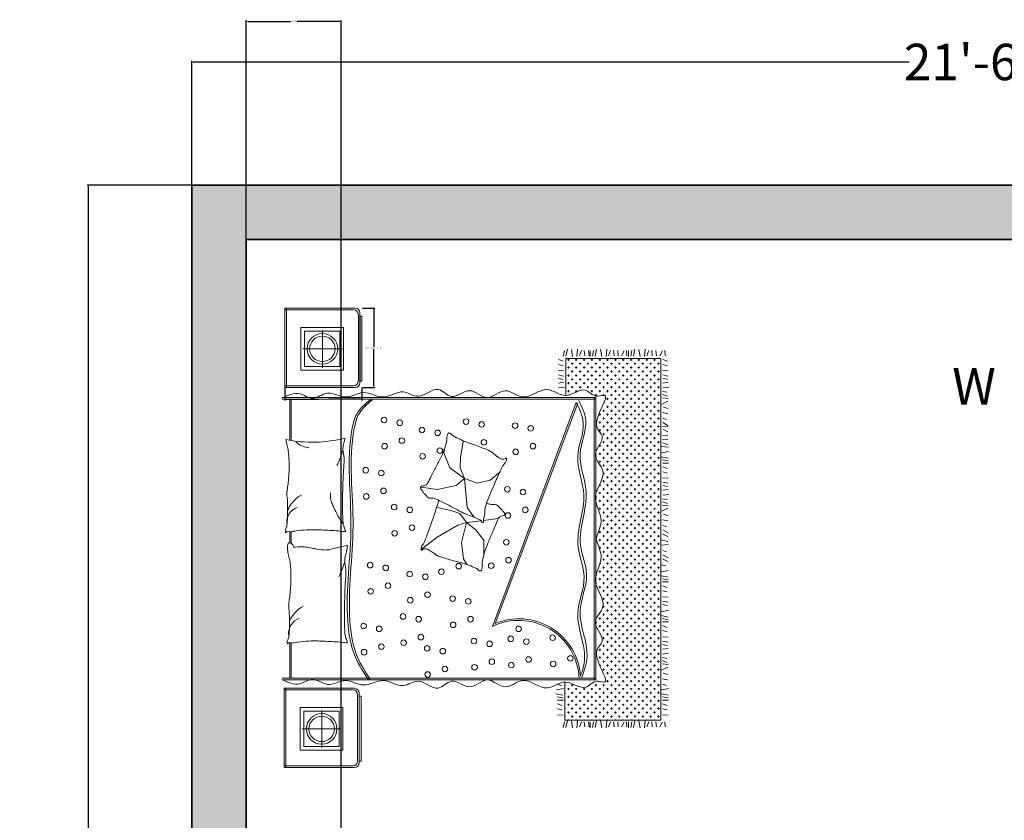
# Model space of a CAD drawing. Units: inches. Extents: x -5 to 330, y -522 to 40.
# Tile 21 of 23: x -5 to 158, y -92 to 40. Entities that reach past the tile are written whole.
import ezdxf

# ---------------------------------------------------------------- set-up
doc = ezdxf.new("R2010")
doc.units = ezdxf.units.IN
doc.header["$MEASUREMENT"] = 0
for name, color, linetype, lineweight in [('A-ANNO-DIMS', 2, 'Continuous', 18), ('A-ANNO-TEXT', 7, 'Continuous', 18), ('A-FURN', 8, 'Continuous', 18), ('A-FURN-PATT', 9, 'Continuous', 13), ('A-WALL', 7, 'Continuous', 35)]:
    doc.layers.add(name, color=color, linetype=linetype, lineweight=lineweight)
doc.layers.add('A-WALL-PATT', color=18, linetype='Continuous', lineweight=13, true_color=0x000000)
doc.styles.get("Standard").update_dxf_attribs({"font": 'arial.ttf'})
doc.dimstyles.get("Standard").update_dxf_attribs({"dimtxt": 0.18, "dimasz": 0.18, "dimexe": 0.18, "dimexo": 0.0625, "dimgap": 0.09, "dimtad": 0, "dimtih": 1, "dimtoh": 1, "dimdec": 0, "dimzin": 0, "dimdsep": 46, "dimlunit": 3, "dimtxsty": 'Standard', "dimcen": 0.09, "dimadec": 0, "dimazin": 0, "dimtfac": 1, "dimtdec": 0, "dimtofl": 0, "dimtmove": 0, "dimatfit": 3, "dimfxl": 1, "dimtolj": 1, "dimtzin": 0, "dimarcsym": 0})

# ---------------------------------------------------------------- blocks, each defined once
blk = doc.blocks.new('*D1')
at = {"layer": 'A-ANNO-DIMS', "color": 0, "lineweight": -2, "transparency": 16777216}
for p, q in [((23.51, 12.42), (23.51, 32.82)), ((23.69, 32.64), (141.81, 32.64)), ((280.83, 32.64), (162.71, 32.64)), ((281.01, 12.42), (281.01, 32.82))]:
    blk.add_line(p, q, dxfattribs=at)
at = {"layer": 'A-ANNO-DIMS', "color": 0, "transparency": 16777216}
for points in [[(23.69, 32.67), (23.69, 32.61), (23.51, 32.64)], [(280.83, 32.67), (280.83, 32.61), (281.01, 32.64)]]:
    blk.add_solid(points, dxfattribs=at)
at = {"layer": 'Defpoints', "color": 0, "transparency": 16777216}
for p in [(281.01, 32.64), (23.51, 12.36), (281.01, 12.36)]:
    blk.add_point(p, dxfattribs=at)
at = {"layer": 'A-ANNO-DIMS', "color": 0, "transparency": 16777216, "insert": (152.26, 32.64), "char_height": 6, "attachment_point": 5}
blk.add_mtext('\\A1;21\'-6"', dxfattribs=at)
blk = doc.blocks.new('*D2')
at = {"layer": 'A-ANNO-DIMS', "color": 0, "lineweight": -2, "transparency": 16777216}
for p, q in [((23.45, 12.36), (6.27, 12.36)), ((6.45, 12.18), (6.45, -203.74)), ((6.45, -425.96), (6.45, -210.05)), ((23.45, -426.14), (6.27, -426.14))]:
    blk.add_line(p, q, dxfattribs=at)
at = {"layer": 'A-ANNO-DIMS', "color": 0, "transparency": 16777216}
for points in [[(6.42, 12.18), (6.48, 12.18), (6.45, 12.36)], [(6.42, -425.96), (6.48, -425.96), (6.45, -426.14)]]:
    blk.add_solid(points, dxfattribs=at)
at = {"layer": 'Defpoints', "color": 0, "transparency": 16777216}
for p in [(23.51, 12.36), (6.45, -426.14), (23.51, -426.14)]:
    blk.add_point(p, dxfattribs=at)
at = {"layer": 'A-ANNO-DIMS', "color": 0, "transparency": 16777216, "insert": (6.45, -206.89), "char_height": 6, "attachment_point": 5}
blk.add_mtext('\\A1;36\'-7"', dxfattribs=at)
blk = doc.blocks.new('NIGHTSTAND-13IN')
for p, q in [((0, 0), (0, 13.05)), ((0, 13.05), (11.58, 13.05)), ((0.26, 0), (0.26, 13.05)), ((0, 12.79), (11.32, 12.79)), ((12.1, 12.01), (12.1, 1.03)), ((12.36, 12.27), (12.36, 0.77)), ((9.67, 9.89), (2.61, 9.89)), ((2.61, 2.83), (2.61, 9.89)), ((9.67, 2.83), (9.67, 9.89)), ((9.04, 9.26), (3.24, 9.26)), ((3.24, 3.46), (3.24, 9.26)), ((6.17, 3.23), (6.17, 9.39)), ((9.04, 3.46), (9.04, 9.26)), ((2.96, 6.35), (9.46, 6.35)), ((9.04, 3.46), (3.24, 3.46)), ((9.67, 2.83), (2.61, 2.83)), ((11.32, 0.26), (0, 0.26)), ((11.58, 0), (0, 0))]:
    blk.add_line(p, q)
blk.add_lwpolyline([(12.38, 11.76), (12.38, 1.04), (12.69, 1.04), (12.69, 11.76)], close=True)
for radius in [2.52, 2.1]:
    blk.add_circle((6.17, 6.35), radius)
for centre, start, end in [((11.58, 12.27), 0, 90), ((11.32, 12.01), 0, 90), ((11.32, 1.03), 270, 0), ((11.58, 0.77), 270, 0)]:
    blk.add_arc(centre, 0.775, start, end)
blk = doc.blocks.new('*D25')
at = {"layer": 'A-ANNO-DIMS', "color": 0, "lineweight": -2, "transparency": 16777216}
for p, q in [((51.65, -7.95), (53.72, -7.95)), ((53.54, -8.13), (53.54, -14.29)), ((53.54, -20.81), (53.54, -14.65)), ((51.65, -20.99), (53.72, -20.99))]:
    blk.add_line(p, q, dxfattribs=at)
at = {"layer": 'A-ANNO-DIMS', "color": 0, "transparency": 16777216}
for points in [[(53.51, -8.13), (53.57, -8.13), (53.54, -7.95)], [(53.51, -20.81), (53.57, -20.81), (53.54, -20.99)]]:
    blk.add_solid(points, dxfattribs=at)
at = {"layer": 'Defpoints', "color": 0, "transparency": 16777216}
for p in [(51.58, -7.95), (53.54, -7.95), (51.58, -20.99)]:
    blk.add_point(p, dxfattribs=at)
at = {"layer": 'A-ANNO-DIMS', "color": 0, "transparency": 16777216, "insert": (53.54, -14.47), "char_height": 0.18, "attachment_point": 5}
blk.add_mtext('\\A1;NIGHTSTAND 1\'-1" TYP.', dxfattribs=at)
blk = doc.blocks.new('*D26')
at = {"layer": 'A-ANNO-DIMS', "color": 0, "lineweight": -2, "transparency": 16777216}
for p, q in [((38.89, -21.05), (38.89, -23.13)), ((51.58, -21.05), (51.58, -23.13)), ((39.07, -22.95), (44.4, -22.95)), ((51.4, -22.95), (46.08, -22.95))]:
    blk.add_line(p, q, dxfattribs=at)
at = {"layer": 'A-ANNO-DIMS', "color": 0, "transparency": 16777216}
for points in [[(39.07, -22.92), (39.07, -22.98), (38.89, -22.95)], [(51.4, -22.92), (51.4, -22.98), (51.58, -22.95)]]:
    blk.add_solid(points, dxfattribs=at)
at = {"layer": 'Defpoints', "color": 0, "transparency": 16777216}
for p in [(38.89, -20.99), (51.58, -20.99), (51.58, -22.95)]:
    blk.add_point(p, dxfattribs=at)
at = {"layer": 'A-ANNO-DIMS', "color": 0, "transparency": 16777216, "insert": (45.24, -22.95), "char_height": 0.18, "attachment_point": 5}
blk.add_mtext('\\A1;1\'-0 1/2" TYP.', dxfattribs=at)
blk = doc.blocks.new('*D43')
at = {"layer": 'A-ANNO-DIMS', "color": 0, "lineweight": -2, "transparency": 16777216}
for p, q in [((32.51, -297.08), (32.51, 39.52)), ((32.69, 39.34), (39.79, 39.34)), ((47.95, 39.34), (40.85, 39.34)), ((48.13, -297.08), (48.13, 39.52))]:
    blk.add_line(p, q, dxfattribs=at)
at = {"layer": 'A-ANNO-DIMS', "color": 0, "transparency": 16777216}
for points in [[(32.69, 39.37), (32.69, 39.31), (32.51, 39.34)], [(47.95, 39.37), (47.95, 39.31), (48.13, 39.34)]]:
    blk.add_solid(points, dxfattribs=at)
at = {"layer": 'Defpoints', "color": 0, "transparency": 16777216}
for p in [(48.13, 39.34), (32.51, -297.14), (48.13, -297.14)]:
    blk.add_point(p, dxfattribs=at)
at = {"layer": 'A-ANNO-DIMS', "color": 0, "transparency": 16777216, "insert": (40.32, 39.34), "char_height": 0.18, "attachment_point": 5}
blk.add_mtext('\\A1;1\'-3 1/2"', dxfattribs=at)

msp = doc.modelspace()

# ---------------------------------------------------------------- hatches: boundary and pattern name
at = {"layer": 'A-FURN-PATT'}
h = msp.add_hatch(dxfattribs=at)
h.set_pattern_fill('CROSS', color=256, scale=2.58433, angle=-90, style=0)
h.set_pattern_definition([(270, (2.9259, -5613.9358), (0.64608249, -0.64608249), [0.32304124, -0.96912373]), (360, (2.7644, -5614.09734), (0.64608249, 0.64608249), [0.32304124, -0.96912373])])
edge = h.paths.add_edge_path()
edge.add_line((100.87, -75.84), (85.03, -75.84))
edge.add_line((85.03, -75.84), (85.03, -69.58))
edge.add_spline(control_points=[(85.03, -69.58), (85.08, -69.58), (86.28, -69.56), (88.27, -71.42), (89.86, -69.09), (93.41, -70.4), (88.82, -65.04), (91.96, -62.62), (90.37, -61.1), (90.13, -60.18)], knot_values=[1896.039366, 1896.039366, 1896.039366, 1896.039366, 1901.133447, 2037.052147, 2110.507177, 2158.377997, 2368.992723, 2430.676444, 2542.061162, 2542.061162, 2542.061162, 2542.061162], degree=3, periodic=0)
edge.add_line((90.13, -60.18), (90.13, -59.44))
edge.add_spline(control_points=[(90.13, -59.44), (90.34, -58.65), (92.37, -56.72), (90.41, -54.57), (90.13, -53.24)], knot_values=[2572.217644, 2572.217644, 2572.217644, 2572.217644, 2670.523569, 2827.764492, 2827.764492, 2827.764492, 2827.764492], degree=3, periodic=0)
edge.add_line((90.13, -53.24), (90.13, -52.16))
edge.add_spline(control_points=[(90.13, -52.16), (90.33, -51.08), (91.68, -49), (90.44, -46.95), (90.18, -45.95)], knot_values=[2870.498313, 2870.498313, 2870.498313, 2870.498313, 2999.108306, 3118.80064, 3118.80064, 3118.80064, 3118.80064], degree=3, periodic=0)
edge.add_spline(control_points=[(90.18, -45.95), (90.44, -44.95), (91.68, -42.9), (90.33, -40.82), (90.13, -39.74)], knot_values=[2870.498313, 2870.498313, 2870.498313, 2870.498313, 2990.190647, 3118.80064, 3118.80064, 3118.80064, 3118.80064], degree=3, periodic=0)
edge.add_line((90.13, -39.74), (90.13, -38.66))
edge.add_spline(control_points=[(90.13, -38.66), (90.41, -37.33), (92.37, -35.17), (90.34, -33.24), (90.13, -32.46)], knot_values=[2572.217644, 2572.217644, 2572.217644, 2572.217644, 2729.458567, 2827.764492, 2827.764492, 2827.764492, 2827.764492], degree=3, periodic=0)
edge.add_line((90.13, -32.46), (90.13, -31.72))
edge.add_spline(control_points=[(90.13, -31.72), (90.37, -30.79), (91.96, -29.28), (88.82, -26.86), (93.41, -21.5), (89.86, -22.8), (88.28, -20.49), (86.36, -22.27), (85.2, -22.32)], knot_values=[1902.697505, 1902.697505, 1902.697505, 1902.697505, 2014.082222, 2075.765943, 2286.38067, 2334.251489, 2407.70652, 2542.061162, 2542.061162, 2542.061162, 2542.061162], degree=3, periodic=0)
edge.add_line((85.2, -22.32), (85.2, -16.25))
edge.add_line((85.2, -16.25), (100.87, -16.25))
edge.add_line((100.87, -16.25), (100.87, -75.84))
at = {"layer": 'A-WALL-PATT'}
h = msp.add_hatch(color=256, dxfattribs=at)
h.dxf.hatch_style = 1
h.paths.add_polyline_path([(164.01, -44.15), (159.51, -44.15), (159.51, -153.14), (164.01, -153.14)], flags=17)
h.paths.add_polyline_path([(224.01, -188.14), (272.01, -188.14), (272.01, -218.14), (260.01, -218.14), (260.01, -222.64), (272.01, -222.64), (272.01, -292.64), (159.01, -292.64), (159.01, -297.14), (272.01, -297.14), (272.01, -417.14), (245.51, -417.14), (245.51, -426.14), (272.01, -426.14), (272.01, -495.14), (281.01, -495.14), (281.01, 12.36), (23.51, 12.36), (23.51, -426.14), (62.92, -426.14), (62.92, -417.14), (32.51, -417.14), (32.51, -297.14), (48.13, -297.14), (48.13, -292.64), (32.51, -292.64), (32.51, -140.64), (133.51, -140.64), (133.51, -131.64), (32.51, -131.64), (32.51, 3.36), (159.51, 3.36), (164.01, 3.36), (220.01, 3.36), (224.51, 3.36), (272.01, 3.36), (272.01, -179.14), (159.51, -179.14), (159.51, -188.14), (219.51, -188.14), (219.51, -266.64), (224.01, -266.64), (224.01, -222.64), (236.01, -222.64), (236.01, -218.14), (224.01, -218.14)])
h.paths.add_polyline_path([(133.01, -292.64), (128.51, -292.64), (128.51, -297.14), (128.51, -417.14), (122.92, -417.14), (122.92, -426.14), (133.01, -426.14)], flags=17)
h.paths.add_polyline_path([(185.51, -417.14), (159.01, -417.14), (159.01, -426.14), (185.51, -426.14)], flags=17)
h.paths.add_polyline_path([(133.51, -140.64), (129.01, -140.64), (129.01, -246.64), (133.51, -246.64)], flags=17)
h.paths.add_polyline_path([(246.01, -48.64), (224.51, -48.64), (224.51, -27.63), (220.01, -27.63), (220.01, -48.64), (198.6, -48.64), (198.6, -53.14), (246.01, -53.14)], flags=17)

# ---------------------------------------------------------------- linework, layer by layer
at = {"layer": 'A-FURN'}
for p, q in [((84.79, -15.84), (84.97, -14.9)), ((85.21, -15.84), (85.46, -14.69)), ((86.31, -15.91), (86.12, -14.76)), ((87.04, -15.91), (87.15, -14.69)), ((87.43, -15.77), (87.77, -14.9)), ((88.33, -15.77), (88.25, -14.9)), ((89.03, -15.77), (88.94, -14.9)), ((89.24, -15.91), (89.24, -14.94)), ((89.61, -15.84), (89.79, -14.9)), ((90.03, -15.84), (90.28, -14.69)), ((91.13, -15.91), (90.94, -14.76)), ((91.85, -15.91), (91.97, -14.69)), ((92.25, -15.77), (92.58, -14.9)), ((93.15, -15.77), (93.07, -14.9)), ((93.84, -15.77), (93.76, -14.9)), ((94.38, -15.77), (94.83, -14.97)), ((95.28, -15.77), (95.2, -14.9)), ((95.55, -15.91), (95.55, -14.94)), ((95.92, -15.84), (96.1, -14.9)), ((96.34, -15.84), (96.59, -14.69)), ((97.44, -15.91), (97.25, -14.76)), ((98.16, -15.91), (98.28, -14.69)), ((98.56, -15.77), (98.89, -14.9)), ((99.46, -15.77), (99.38, -14.9)), ((100.15, -15.77), (100.07, -14.9)), ((100.69, -15.77), (101.14, -14.97)), ((101.59, -15.77), (101.51, -14.9)), ((84.75, -16.7), (83.99, -16.4)), ((84.75, -17.43), (83.99, -17.23)), ((85.2, -16.25), (100.87, -16.25)), ((85.2, -22.32), (85.2, -16.25)), ((100.87, -16.25), (100.87, -75.84)), ((101.96, -16.7), (101.2, -16.4)), ((101.96, -17.43), (101.2, -17.23)), ((84.89, -18.28), (83.99, -18.23)), ((84.82, -19.12), (83.99, -18.95)), ((102.1, -18.28), (101.2, -18.23)), ((102.03, -19.12), (101.2, -18.95)), ((84.75, -19.68), (83.99, -19.5)), ((84.89, -20.16), (83.99, -20.28)), ((84.96, -20.95), (83.99, -21.09)), ((101.96, -19.68), (101.2, -19.5)), ((102.1, -20.16), (101.2, -20.28)), ((102.17, -20.95), (101.2, -21.09)), ((38.44, -22.69), (90.13, -22.69)), ((89.87, -22.69), (89.87, -69.21)), ((90.13, -22.69), (90.13, -69.21)), ((101.89, -21.8), (101.16, -21.67)), ((101.96, -22.46), (101.16, -22.16)), ((102.1, -22.83), (101.16, -22.71)), ((38.44, -22.95), (90.13, -22.95)), ((39.67, -22.95), (39.67, -29.73)), ((39.93, -22.95), (39.93, -29.77)), ((86.93, -23.48), (73.09, -60.41)), ((87.17, -23.57), (73.55, -59.92)), ((102.03, -23.25), (101.02, -23.74)), ((102.1, -24.47), (101.3, -24.23)), ((102.02, -25.33), (101.17, -25.14)), ((102.02, -27.43), (101.16, -27.51)), ((101.83, -26.29), (101.2, -26.08)), ((102.1, -27.31), (101.2, -26.8)), ((102.02, -28.87), (101.16, -28.95)), ((102.02, -28.33), (101.23, -27.88)), ((67.85, -32.49), (68.29, -29.96)), ((68.29, -29.96), (68.46, -29.87)), ((102.16, -30.86), (100.94, -30.74)), ((102.02, -29.56), (101.16, -29.64)), ((102.02, -30.46), (101.16, -30.13)), ((65.09, -31.78), (65.18, -31.16)), ((66.07, -34.23), (65.09, -31.78)), ((102.09, -32.68), (100.94, -32.43)), ((102.16, -31.58), (101.01, -31.77)), ((67.76, -34.27), (67.85, -32.49)), ((102.09, -33.1), (101.16, -32.92)), ((102.16, -33.47), (101.2, -33.47)), ((101.96, -34.38), (101.2, -34.08)), ((68.47, -36.01), (66.07, -34.23)), ((68.47, -36.01), (67.76, -34.27)), ((72.74, -36.27), (74.35, -34.89)), ((101.96, -35.11), (101.2, -34.91)), ((63.98, -37.83), (67.14, -37.16)), ((67.14, -37.16), (68.47, -36.01)), ((68.47, -36.01), (68.96, -40.81)), ((68.47, -36.01), (70.6, -36.81)), ((70.6, -36.81), (72.74, -36.27)), ((102.1, -35.96), (101.2, -35.91)), ((102.03, -36.8), (101.2, -36.63)), ((101.96, -37.36), (101.2, -37.18)), ((61.32, -37.47), (63.98, -37.83)), ((102.1, -37.84), (101.2, -37.96)), ((102.17, -38.63), (101.2, -38.77)), ((101.89, -39.48), (101.16, -39.36)), ((101.96, -40.14), (101.16, -39.84)), ((102.1, -40.51), (101.16, -40.39)), ((66.25, -41.28), (63.96, -40.77)), ((67.74, -41.79), (66.25, -41.28)), ((68.81, -43.27), (67.74, -41.79)), ((68.45, -41.77), (69.91, -42.36)), ((68.96, -40.81), (69.89, -42.1)), ((69.89, -42.1), (70.11, -42.41)), ((102.03, -40.93), (101.02, -41.42)), ((102.1, -42.15), (101.3, -41.91)), ((64.01, -45.67), (67.38, -43.73)), ((67.38, -43.73), (68.81, -43.27)), ((68.81, -43.27), (67.99, -46.59)), ((68.81, -43.27), (71.24, -42.97)), ((68.81, -43.27), (70.44, -44.55)), ((69.91, -42.36), (71.03, -42.82)), ((71.62, -42.92), (74.06, -42.62)), ((102.02, -43.01), (101.17, -42.82)), ((101.83, -43.97), (101.2, -43.76)), ((39.67, -44.8), (39.67, -46.6)), ((39.93, -44.8), (39.93, -46.7)), ((70.44, -44.55), (71.67, -46.24)), ((102.02, -45.58), (101.16, -45.18)), ((102.1, -44.99), (101.2, -44.48)), ((49.14, -47.02), (48.36, -47.21)), ((61.32, -47.72), (64.01, -45.67)), ((67.99, -46.59), (68.35, -49.25)), ((71.67, -46.24), (71.67, -48.64)), ((102.03, -46.39), (100.95, -46.14)), ((102.1, -46.87), (101.02, -46.99)), ((48.36, -47.21), (46.23, -47.74)), ((101.83, -48.08), (101.2, -47.86)), ((102.1, -49.09), (101.2, -48.59)), ((68.35, -49.25), (68.87, -50.18)), ((101.68, -50.41), (100.95, -50.25)), ((102.02, -49.69), (101.16, -49.28)), ((102.13, -51.19), (100.98, -51.38)), ((102.06, -52.28), (100.91, -52.04)), ((102.06, -52.7), (101.12, -52.53)), ((102.13, -53.07), (101.16, -53.07)), ((101.93, -53.99), (101.16, -53.68)), ((101.93, -54.71), (101.16, -54.51)), ((102.07, -55.56), (101.16, -55.51)), ((102, -56.41), (101.16, -56.24)), ((101.93, -56.96), (101.16, -56.78)), ((102.13, -57.77), (100.98, -57.96)), ((102.06, -58.86), (100.91, -58.62)), ((102.06, -59.29), (101.12, -59.11)), ((102.13, -59.65), (101.16, -59.65)), ((101.93, -60.57), (101.16, -60.27)), ((101.93, -61.3), (101.16, -61.09)), ((39.67, -63.05), (39.67, -68.95)), ((39.93, -63.12), (39.93, -68.95)), ((102.07, -62.14), (101.16, -62.1)), ((102, -62.99), (101.16, -62.82)), ((101.93, -63.54), (101.16, -63.37)), ((102.07, -64.02), (101.16, -64.15)), ((102.14, -64.81), (101.16, -64.95)), ((101.86, -65.67), (101.12, -65.54)), ((101.93, -66.33), (101.12, -66.02)), ((102, -67.12), (100.99, -67.61)), ((102.07, -66.69), (101.12, -66.57)), ((102.07, -68.34), (101.27, -68.09)), ((38.44, -68.95), (90.13, -68.95)), ((38.44, -69.21), (90.13, -69.21)), ((85.03, -75.84), (85.03, -69.58)), ((101.99, -69.2), (101.13, -69.01)), ((84.8, -70.65), (83.65, -70.83)), ((84.47, -70.16), (83.84, -69.94)), ((102.13, -70.65), (100.98, -70.83)), ((101.79, -70.16), (101.16, -69.94)), ((84.73, -71.74), (83.58, -71.49)), ((84.73, -72.16), (83.8, -71.99)), ((84.8, -72.53), (83.84, -72.53)), ((102.06, -71.74), (100.91, -71.49)), ((102.06, -72.16), (101.12, -71.99)), ((102.13, -72.53), (101.16, -72.53)), ((84.61, -73.44), (83.84, -73.14)), ((84.61, -74.17), (83.84, -73.97)), ((101.93, -73.44), (101.16, -73.14)), ((101.93, -74.17), (101.16, -73.97)), ((84.74, -75.02), (83.84, -74.97)), ((84.79, -77.03), (84.97, -76.1)), ((100.87, -75.84), (85.03, -75.84)), ((85.21, -77.03), (85.46, -75.88)), ((86.31, -77.1), (86.12, -75.95)), ((87.04, -77.1), (87.15, -75.88)), ((87.43, -76.96), (87.77, -76.1)), ((88.33, -76.96), (88.25, -76.1)), ((89.03, -76.96), (88.94, -76.1)), ((89.24, -77.1), (89.24, -76.14)), ((89.61, -77.03), (89.79, -76.1)), ((90.03, -77.03), (90.28, -75.88)), ((91.13, -77.1), (90.94, -75.95)), ((91.85, -77.1), (91.97, -75.88)), ((92.25, -76.96), (92.58, -76.1)), ((93.15, -76.96), (93.07, -76.1)), ((93.84, -76.96), (93.76, -76.1)), ((94.38, -76.96), (94.83, -76.17)), ((95.28, -76.96), (95.2, -76.1)), ((95.55, -77.1), (95.55, -76.14)), ((95.92, -77.03), (96.1, -76.1)), ((96.34, -77.03), (96.59, -75.88)), ((97.44, -77.1), (97.25, -75.95)), ((98.16, -77.1), (98.28, -75.88)), ((98.56, -76.96), (98.89, -76.1)), ((99.46, -76.96), (99.38, -76.1)), ((100.15, -76.96), (100.07, -76.1)), ((100.69, -76.96), (101.14, -76.17)), ((102.07, -75.02), (101.16, -74.97)), ((101.59, -76.96), (101.51, -76.1))]:
    msp.add_line(p, q, dxfattribs=at)
for centre in [(55.23, -26.37), (57.81, -26.83), (61.48, -28.02), (68.75, -26.64), (71.32, -27.1), (76.84, -27.29), (79.41, -27.75), (64.06, -28.48), (55.32, -30.69), (58.17, -29.77), (71.69, -30.05), (79.78, -30.69), (61.58, -32.35), (64.43, -31.43), (76.93, -31.61), (52.2, -34.65), (54.77, -35.11), (75.57, -37.79), (52.29, -38.97), (55.14, -38.05), (78.14, -38.25), (56.89, -40.72), (59.46, -41.18), (75.66, -42.11), (78.51, -41.19), (59.83, -44.12), (56.98, -45.04), (75.39, -46.53), (52.93, -50.29), (55.51, -50.75), (67.53, -50.46), (72.9, -50.39), (75.75, -49.47), (59.46, -51.76), (62.04, -52.22), (64.68, -51.38), (55.88, -53.69), (53.03, -54.61), (62.4, -55.16), (59.55, -56.08), (66.54, -55.81), (69.11, -56.27), (58.36, -58.75), (51.85, -60.33), (60.93, -59.21), (66.63, -60.13), (69.48, -59.21), (54.43, -60.79), (61.3, -62.16), (77.41, -60.79), (54.79, -63.73), (58.45, -63.08), (70.05, -62.81), (72.63, -63.27), (76.12, -62.44), (78.7, -62.9), (83.02, -62.26), (51.94, -64.65), (62.33, -64.01), (64.91, -64.47), (73, -66.21), (76.21, -66.77), (79.06, -65.85), (83.11, -66.58), (85.96, -65.66), (62.42, -68.33), (65.27, -67.41), (70.15, -67.13)]:
    msp.add_circle(centre, 0.46, dxfattribs=at)
for centre, radius, start, end in [((67.14, -29.31), 1.55, 166.9598, 183.3881), ((66.91, -29.26), 1.32, 148.3083, 166.9598), ((65.92, -28.65), 0.15, 90.9614, 148.3083), ((65.92, -28.93), 0.433, 40.5086, 90.9614), ((67.74, -27.38), 1.95, 220.5086, 243.6668), ((97.39, 32.52), 68.79, 243.6668, 244.8268), ((43.36, -7.71), 22.32, 258.8097, 284.0422), ((46.82, -28.45), 7.88, 188.4372, 195.744), ((33.22, -32.29), 6.26, 7.5469, 15.744), ((43.22, -27.37), 3.62, 224.9024, 264.3689), ((52.21, -31.16), 3.77, 173.5659, 191.5586), ((51.54, -31.09), 3.09, 162.6136, 173.5659), ((42.92, -28.39), 5.94, 342.6136, 350.5159), ((54.71, -27.42), 11.11, 339.2514, 347.3748), ((63.97, -29.5), 1.63, 347.3748, 3.3881), ((70.1, -25.53), 4.65, 244.8268, 249.2919), ((73.44, -16.69), 14.1, 249.2919, 251.7631), ((55.7, -70.53), 42.59, 70.3416, 71.7631), ((52.62, -79.17), 51.76, 67.7645, 70.3416), ((21.93, -33.78), 17.64, 0, 7.5469), ((30.21, -25.72), 19.09, 334.6889, 342.8018), ((42.69, -33.11), 5.95, 357.2509, 11.5586), ((50.03, -25.65), 16.12, 332.5079, 339.2514), ((70.28, -35.95), 5.08, 59.5306, 67.7645), ((71.8, -33.38), 2.09, 45.9036, 59.5306), ((76.74, -28.28), 5.01, 225.9036, 234.6985), ((79.1, -24.94), 9.1, 234.6985, 238.7862), ((12.47, -33.78), 27.11, 353.9133, 0), ((12.37, -31.65), 36.3, 355.3824, 357.2509), ((203.32, -107.58), 157.69, 152.1518, 152.5001), ((-69.51, 36.56), 150.88, 332.1518, 332.5079), ((94.03, -43.87), 21.63, 152.8972, 155.4754), ((74.92, -31.85), 1.02, 238.7862, 251.0332), ((74.71, -32.44), 0.395, 251.0332, 268.3327), ((74.76, -30.84), 1.99, 268.3327, 276.0115), ((76.6, -34.94), 2.05, 137.0187, 152.8972), ((74.93, -32.46), 0.366, 276.0115, 319.0249), ((73.96, -32.49), 1.55, 317.0187, 335.2589), ((75.33, -32.81), 0.163, 72.3233, 139.0249), ((75.34, -32.76), 0.115, 359.5525, 72.3233), ((74.55, -32.76), 0.911, 335.2589, 359.5525), ((135.29, -39.63), 86.89, 177.3904, 179.0296), ((79.89, -37.11), 31.44, 175.3824, 177.3904), ((-8.68, -0.04), 80.04, 332.7098, 333.5853), ((109.67, -58.83), 52.11, 152.5001, 153.5853), ((194.13, -89.53), 131.65, 155.4754, 156.5205), ((25.82, -35.21), 13.68, 349.8101, 353.9133), ((61.55, -37.57), 0.329, 86.7545, 218.8136), ((61.63, -36.32), 0.927, 266.7545, 332.7098), ((147.92, -69.46), 81.28, 156.5205, 158.9957), ((43.16, -38.33), 3.94, 169.8101, 177.4614), ((46.7, -38.48), 7.49, 177.4614, 184.8018), ((43.62, -43.54), 5.17, 113.0028, 118.3168), ((53.42, -38.83), 7.03, 176.4448, 184.0828), ((196.17, -40.66), 147.79, 179.0296, 180.2865), ((62.7, -36.65), 1.8, 218.8136, 224.1274), ((60.57, -38.72), 1.17, 37.5287, 44.1274), ((53.66, -44.03), 9.89, 36.2163, 37.5287), ((75.4, -28.1), 17.07, 216.2163, 217.2151), ((66.29, -35.02), 5.62, 217.2151, 223.5224), ((63.66, -37.52), 2, 223.5224, 234.1064), ((16.76, -41), 22.57, 0.5757, 4.8018), ((41.36, -41.57), 1.98, 141.6114, 152.7604), ((47.74, -46.62), 10.12, 136.1885, 141.6114), ((44.64, -43.64), 5.82, 129.0349, 136.1885), ((41.77, -40.11), 1.27, 118.3168, 129.0349), ((47.9, -39.22), 1.5, 184.0828, 200.6743), ((58.75, -35.13), 13.09, 200.6743, 204.3265), ((80.55, -25.28), 37.01, 204.3265, 206.4985), ((62.83, -38.67), 0.584, 234.1064, 278.0492), ((63.08, -40.42), 1.18, 67.5838, 98.0492), ((-13.74, -16.68), 81.28, 340.9164, 343.3915), ((53.62, -63.34), 25.98, 64.9471, 67.5838), ((61.26, -39.05), 3.01, 343.3915, 349.2634), ((46.16, -79.29), 43.59, 62.9116, 64.9471), ((47.6, -76.5), 40.45, 60.064, 62.9116), ((74.86, -41.41), 3.01, 158.9957, 171.8784), ((80.75, -15.56), 25.98, 250.6552, 251.9797), ((73.08, -39.14), 1.18, 251.9797, 282.4451), ((73.46, -40.87), 0.584, 58.5023, 102.4451), ((72.72, -42.08), 2, 47.9183, 58.5023), ((41.73, -43.2), 2.56, 108.4397, 184.2159), ((0.71, -41.16), 38.62, 358.0921, 0.5757), ((44.98, -43.43), 6.05, 152.7604, 159.1397), ((54.65, -38.19), 8.08, 206.4985, 212.135), ((78.47, -41.25), 30.08, 180.2865, 183.574), ((70.55, -36.64), 5.54, 240.064, 247.7645), ((67.26, -41.13), 4.64, 345.1193, 352.3216), ((70.03, -41.51), 1.84, 352.3216, 4.5118), ((73.57, -41.23), 1.71, 171.8784, 184.5118), ((74.84, -43.12), 0.927, 91.1504, 157.1056), ((70.29, -44.77), 5.62, 41.611, 47.9183), ((61.74, -52.37), 17.07, 40.6122, 41.611), ((82.2, -34.82), 9.89, 220.6122, 221.9246), ((74.82, -41.86), 0.329, 271.1504, 43.2095), ((75.71, -40.65), 1.17, 221.9246, 228.5233), ((73.75, -42.87), 1.8, 43.2095, 48.5233), ((37.84, -43.56), 1.39, 329.3487, 354.7408), ((18.1, -41.74), 21.21, 354.7408, 358.0921), ((63.76, -32.47), 18.83, 212.135, 215.8263), ((52.21, -42.89), 3.77, 183.574, 192.869), ((49.68, -43.47), 1.17, 192.869, 207.2841), ((-61.35, -0.21), 131.65, 339.8713, 340.9164), ((70.8, -43.37), 0.596, 17.1867, 67.7645), ((71.49, -43.16), 0.121, 197.1867, 340.6201), ((71.38, -43.12), 0.238, 340.6201, 4.2593), ((72.49, -43.04), 0.878, 172.0178, 184.2593), ((76.62, -43.62), 5.05, 165.1193, 172.0178), ((147.73, -73.9), 80.04, 157.1056, 157.9812), ((39.68, -44.65), 0.746, 149.3487, 184.3025), ((39.58, -44.65), 0.649, 184.3025, 201.7883), ((39.06, -44.86), 0.0884, 201.7883, 250.436), ((39.05, -44.89), 0.0599, 250.436, 11.8931), ((39.22, -44.85), 0.111, 111.9904, 191.8931), ((39.33, -45.12), 0.403, 68.579, 111.9904), ((39.78, -43.96), 0.847, 248.579, 278.1335), ((39, -38.51), 6.36, 278.1335, 282.1095), ((41.41, -49.73), 5.13, 97.6809, 102.1095), ((43.88, -68.04), 23.6, 93.3687, 97.6809), ((43.53, -61.99), 17.54, 88.3669, 93.3687), ((43.02, -79.73), 35.28, 86.945, 88.3669), ((26.12, -396.38), 352.39, 86.4951, 86.945), ((47.16, -52.94), 8.3, 80.0016, 86.4951), ((48.68, -44.27), 0.5, 260.0016, 286.6978), ((46.87, -44.92), 1.98, 16.2212, 27.2841), ((46.61, -44.99), 2.26, 7.1204, 16.2212), ((48.82, -44.72), 0.0341, 286.6978, 7.1204), ((-71.9, 17.08), 157.69, 336.5477, 336.896), ((25.22, -24.35), 52.11, 336.896, 337.9812), ((41.63, -47.33), 2.34, 168.7276, 180), ((39.67, -46.94), 0.339, 63.4195, 168.7276), ((39.43, -47.42), 0.883, 4.4002, 63.4195), ((42.19, -46.54), 7, 350.5159, 355.9171), ((49.14, -47.04), 0.0237, 355.9171, 104.0449), ((62.83, -47.88), 1.55, 141.4146, 159.6548), ((60.02, -45.64), 2.05, 321.4146, 337.2931), ((41.95, -38.08), 21.63, 337.2931, 339.8713), ((87.22, -52.86), 16.12, 156.9038, 163.6473), ((211.18, -105.73), 150.88, 156.5477, 156.9038), ((43.46, -47.33), 4.16, 180, 188.4372), ((47.13, -46.78), 7.88, 188.4372, 195.744), ((41.68, -59.99), 12.71, 90, 96.2324), ((41.68, -52.55), 5.27, 80.3156, 90), ((38.73, -69.82), 22.79, 77.8016, 80.3156), ((45.28, -39.53), 8.2, 257.8016, 261.9949), ((46.51, -30.79), 17.03, 261.9949, 267.3351), ((45.8, -46.05), 1.75, 267.3351, 284.0452), ((51.85, -49.42), 3.09, 162.6136, 173.5659), ((43.23, -46.72), 5.94, 342.6136, 350.5159), ((61.45, -47.67), 0.163, 183.9524, 323.4208), ((62.23, -47.66), 0.911, 159.6548, 183.9484), ((61.87, -47.98), 0.366, 100.4074, 143.4208), ((62.17, -49.58), 1.99, 92.7286, 100.4074), ((62.09, -47.99), 0.395, 75.4291, 92.7286), ((61.93, -48.59), 1.02, 63.1821, 75.4291), ((58.29, -55.8), 9.1, 59.0944, 63.1821), ((60.39, -52.29), 5.01, 50.2995, 59.0944), ((64.93, -46.83), 2.09, 230.2995, 243.9265), ((66.24, -44.15), 5.08, 243.9265, 252.1604), ((82.42, -51.46), 11.11, 163.6473, 171.7707), ((33.52, -50.62), 6.26, 7.5469, 15.744), ((22.24, -52.11), 17.64, 0, 7.5469), ((30.52, -44.05), 19.09, 334.6889, 342.8018), ((52.52, -49.49), 3.77, 173.5659, 191.5586), ((43, -51.44), 5.95, 357.2509, 11.5586), ((80.54, 0.3), 51.76, 252.1604, 254.7375), ((78.13, -8.55), 42.59, 254.7375, 256.159), ((64.56, -63.59), 14.1, 73.6878, 76.159), ((67.22, -54.52), 4.65, 69.2227, 73.6878), ((44.46, -114.5), 68.79, 68.0627, 69.2227), ((73.03, -50.1), 1.63, 171.7707, 187.784), ((69.88, -50.53), 1.55, 351.3557, 7.784), ((12.68, -49.98), 36.3, 355.3824, 357.2509), ((69.43, -52.5), 1.95, 44.9045, 68.0627), ((71.12, -50.82), 0.433, 224.9045, 275.3572), ((71.15, -51.1), 0.15, 275.3572, 332.7041), ((70.11, -50.56), 1.32, 332.7041, 351.3557), ((12.77, -52.11), 27.11, 353.9133, 0), ((80.2, -55.44), 31.44, 175.3824, 177.3904), ((26.13, -53.54), 13.68, 349.8101, 353.9133), ((135.6, -57.96), 86.89, 177.3904, 179.0296), ((43.47, -56.65), 3.94, 169.8101, 177.4614), ((47.01, -56.81), 7.49, 177.4614, 184.8018), ((196.48, -58.99), 147.79, 179.0296, 180.2865), ((17.06, -59.33), 22.57, 0.5757, 4.8018), ((48.05, -64.95), 10.12, 136.1885, 141.6114), ((44.94, -61.97), 5.82, 129.0349, 136.1885), ((42.08, -58.44), 1.27, 118.3168, 129.0349), ((43.93, -61.87), 5.17, 113.0028, 118.3168), ((42.04, -61.53), 2.56, 108.4397, 184.2159), ((1.01, -59.49), 38.62, 358.0921, 0.5757), ((45.28, -61.76), 6.05, 152.7604, 159.1397), ((41.67, -59.9), 1.98, 141.6114, 152.7604), ((78.78, -59.58), 30.08, 180.2865, 183.574), ((77.46, -69.34), 9.94, 2.2326, 116.0937), ((77.46, -69.34), 10.2, 4.2507, 112.5558), ((18.41, -60.07), 21.21, 354.7408, 358.0921), ((52.52, -61.22), 3.77, 183.574, 192.869), ((39.99, -62.98), 0.746, 149.3487, 184.3025), ((39.89, -62.98), 0.649, 184.3025, 201.7883), ((39.37, -63.19), 0.0884, 201.7883, 250.436), ((38.15, -61.88), 1.39, 329.3487, 354.7408), ((39.36, -63.22), 0.0599, 250.436, 11.8931), ((39.53, -63.18), 0.111, 111.9904, 191.8931), ((39.64, -63.45), 0.403, 68.579, 111.9904), ((40.09, -62.29), 0.847, 248.579, 278.1335), ((39.31, -56.83), 6.36, 278.1335, 282.1095), ((41.72, -68.06), 5.13, 97.6809, 102.1095), ((44.19, -86.37), 23.6, 93.3687, 97.6809), ((43.83, -80.32), 17.54, 88.3669, 93.3687), ((43.33, -98.06), 35.28, 86.945, 88.3669), ((26.43, -414.71), 352.39, 86.4951, 86.945), ((47.46, -71.27), 8.3, 80.0016, 86.4951), ((49.99, -61.8), 1.17, 192.869, 207.2841), ((48.99, -62.6), 0.5, 260.0016, 286.6978), ((47.18, -63.25), 1.98, 16.2212, 27.2841), ((46.92, -63.32), 2.26, 7.1204, 16.2212), ((49.13, -63.05), 0.0341, 286.6978, 7.1204)]:
    msp.add_arc(centre, radius, start, end, dxfattribs=at)
for points, knots in [([(38.35, -22.78), (39.36, -22.3), (41.08, -21.47), (43.55, -23.41), (46.01, -21.2), (48.88, -23.29), (51.93, -21.09), (55.14, -23.43), (58.17, -20.97), (61.15, -23.4), (63.92, -20.22), (66.48, -23.48), (69.38, -20.44), (72.25, -23.79), (75.16, -20.52), (78.41, -23.79), (81.83, -20.18), (85.19, -23.36), (88.27, -20.48), (89.86, -22.8), (93.41, -21.5), (88.82, -26.86), (92.07, -29.36), (88.92, -32.05), (92.63, -35.12), (88.84, -38.9), (91.83, -42.65), (90.44, -44.95), (90.18, -45.95)], [0, 0, 0, 0, 119.23822, 203.934156, 305.051348, 423.414205, 538.771408, 673.601551, 801.564672, 901.488314, 1036.739405, 1131.503109, 1252.869042, 1373.114912, 1497.089457, 1612.174498, 1779.078494, 1901.133447, 2037.052147, 2110.507177, 2158.377997, 2368.992723, 2430.676444, 2554.510696, 2670.523569, 2841.287389, 2999.108306, 3118.80064, 3118.80064, 3118.80064, 3118.80064]), ([(52.93, -23.07), (52.08, -23.77), (50.59, -25.01), (48.84, -32.29), (50.62, -43.7), (48.55, -56.25), (49.94, -65.04), (51.84, -67.97), (52.62, -69.17)], [0, 0, 0, 0, 3.207352, 5.642725, 21.784837, 37.406991, 43.551817, 47.803661, 47.803661, 47.803661, 47.803661]), ([(53.28, -23.07), (52.43, -23.77), (50.93, -25.01), (49.18, -32.29), (50.96, -43.7), (48.9, -56.25), (50.28, -65.04), (52.18, -67.97), (52.96, -69.17)], [0, 0, 0, 0, 3.207352, 5.642725, 21.784837, 37.406991, 43.551817, 47.803661, 47.803661, 47.803661, 47.803661]), ([(86.94, -23.52), (87.46, -24.6), (88.83, -27.44), (86.19, -32.58), (89.37, -39.35), (86.08, -46.09), (89.12, -52.6), (85.97, -58.71), (88.96, -64.25), (87.98, -67.62), (87.63, -68.58)], [0, 0, 0, 0, 134.096191, 351.943146, 593.51487, 936.925241, 1129.231545, 1368.385454, 1657.415202, 1773.3935, 1773.3935, 1773.3935, 1773.3935]), ([(87.33, -23.15), (87.86, -24.23), (89.23, -27.07), (86.59, -32.21), (89.77, -38.98), (86.48, -45.72), (89.52, -52.23), (86.37, -58.34), (89.49, -64.14), (88.22, -67.74), (87.76, -68.95)], [0, 0, 0, 0, 134.096191, 351.943146, 593.51487, 936.925241, 1129.231545, 1368.385454, 1657.415202, 1803.02854, 1803.02854, 1803.02854, 1803.02854]), ([(38.35, -69.12), (39.36, -69.6), (41.08, -70.43), (43.55, -68.49), (46.01, -70.7), (48.88, -68.61), (51.93, -70.81), (55.14, -68.47), (58.17, -70.93), (61.15, -68.5), (63.92, -71.68), (66.48, -68.42), (69.38, -71.46), (72.25, -68.1), (75.16, -71.38), (78.41, -68.11), (81.83, -71.71), (85.19, -68.54), (88.27, -71.42), (89.86, -69.09), (93.41, -70.4), (88.82, -65.04), (92.07, -62.54), (88.92, -59.85), (92.63, -56.77), (88.84, -53), (91.83, -49.24), (90.44, -46.95), (90.18, -45.95)], [0, 0, 0, 0, 119.23822, 203.934156, 305.051348, 423.414205, 538.771408, 673.601551, 801.564672, 901.488314, 1036.739405, 1131.503109, 1252.869042, 1373.114912, 1497.089457, 1612.174498, 1779.078494, 1901.133447, 2037.052147, 2110.507177, 2158.377997, 2368.992723, 2430.676444, 2554.510696, 2670.523569, 2841.287389, 2999.108306, 3118.80064, 3118.80064, 3118.80064, 3118.80064])]:
    msp.add_open_spline(points, degree=3, knots=knots, dxfattribs=at)
at = {"layer": 'A-WALL'}
for p, q in [((23.51, 12.36), (23.51, -495.14)), ((23.51, 12.36), (281.01, 12.36)), ((32.51, 3.36), (159.51, 3.36)), ((32.51, 3.36), (32.51, -131.64))]:
    msp.add_line(p, q, dxfattribs=at)

# ---------------------------------------------------------------- block references
at = {"layer": 'A-FURN'}
for p in [(38.89, -20.99), (38.77, -83.64)]:
    msp.add_blockref('NIGHTSTAND-13IN', p, dxfattribs=at)

# ---------------------------------------------------------------- texts
at = {"layer": 'A-ANNO-TEXT', "insert": (148.92, -17.82), "char_height": 6, "attachment_point": 1}
msp.add_mtext('W', dxfattribs=at)

# ---------------------------------------------------------------- dimensions: what is measured, and where the dimension line sits
at = {"layer": 'A-ANNO-DIMS'}
for base, p1, p2, override, picture, middle in [((48.13, 39.34), (32.51, -297.14), (48.13, -297.14), {"dimdec": 1, "dimlfac": 1, "dimrnd": 0, "dimzin": 1, "dimdsep": 46, "dimlunit": 4, "dimfrac": 2}, '*D43', (40.32, 39.34)), ((281.00988858, 32.64453517), (23.50988858, 12.35641797), (281.00988858, 12.35641797), {"dimtxt": 6, "dimclrd": 0, "dimclre": 0, "dimclrt": 0}, '*D1', (152.25988858, 32.64453517))]:
    dim = msp.add_linear_dim(base=base, p1=p1, p2=p2, dimstyle='Standard', override=override, dxfattribs=at)
    dim.commit()
    dim.dimension.update_dxf_attribs({"geometry": picture, "text_midpoint": middle})
dim = msp.add_linear_dim(base=(6.45432189, -426.14358203), p1=(23.50988858, 12.35641797), p2=(23.50988858, -426.14358203), angle=90, dimstyle='Standard', override={"dimtxt": 6, "dimclrd": 0, "dimclre": 0, "dimclrt": 0}, dxfattribs=at)
dim.commit()
dim.dimension.update_dxf_attribs({"geometry": '*D2', "text_midpoint": (6.45432189, -206.89358203)})
dim = msp.add_linear_dim(base=(53.54, -7.95), p1=(51.58, -20.99), p2=(51.58, -7.95), angle=90, text='NIGHTSTAND <> TYP.', dimstyle='Standard', override={"dimdec": 1, "dimlfac": 1, "dimrnd": 0, "dimzin": 1, "dimdsep": 46, "dimlunit": 4, "dimfrac": 2}, dxfattribs=at)
dim.commit()
dim.dimension.update_dxf_attribs({"geometry": '*D25', "text_midpoint": (53.54, -14.47)})
dim = msp.add_linear_dim(base=(51.58, -22.95), p1=(38.89, -20.99), p2=(51.58, -20.99), text='<> TYP.', dimstyle='Standard', override={"dimdec": 1, "dimlfac": 1, "dimrnd": 0, "dimzin": 1, "dimdsep": 46, "dimlunit": 4, "dimfrac": 2}, dxfattribs=at)
dim.commit()
dim.dimension.update_dxf_attribs({"geometry": '*D26', "text_midpoint": (45.24, -22.95)})

doc.saveas('drawing.dxf')
